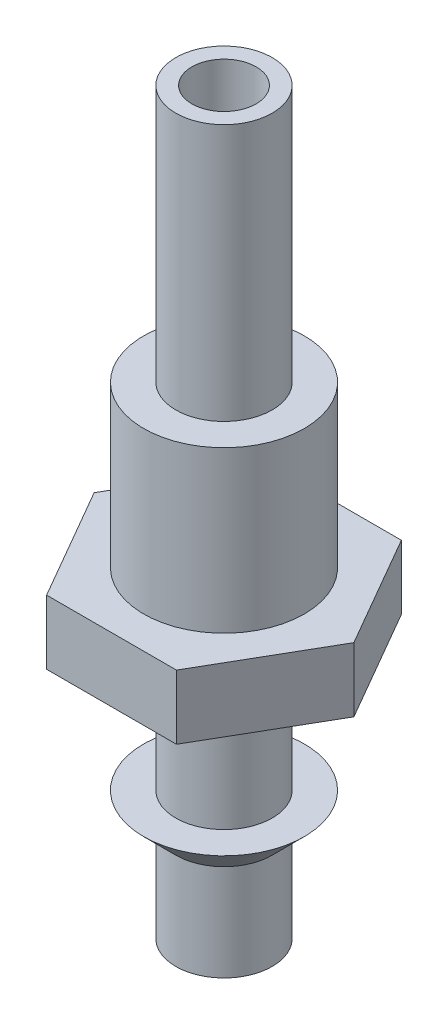
from build123d import *

# Parameters (mm, degrees)
HEX_7AF_DEPTH     = 2
BORE_PROFILE_2_R  = 1
FUEL_BORE_2_DEPTH = 24.613202522


with BuildPart() as part:
    # Lower Spigot Profile → Lower Spigot and Collar (revolve)
    with BuildSketch(Plane.XY, mode=Mode.PRIVATE) as lower_spigot_and_collar_sk:
        Polygon((0, 0), (0, -8), (1.5, -8), (1.5, -5), (2.5, -4), (1.5, -4), (1.5, 0), align=None)
    revolve(lower_spigot_and_collar_sk.sketch.rotate(Axis((0, 0, 0), (0, -1, 0)), 90), axis=Axis((0, 0, 0), (0, -1, 0)))

    # Hex Profile 7AF → Hex 7AF (add)
    with BuildSketch(Plane(origin=(0, 0, 0), x_dir=(1, 0, 0), z_dir=(0, 1, 0))):
        Polygon((4.041451884, 0), (2.020725942, 3.5), (-2.020725942, 3.5), (-4.041451884, 0), (-2.020725942, -3.5), (2.020725942, -3.5), align=None)
    extrude(amount=HEX_7AF_DEPTH)

    # Upper Pipe Profile → Upper Pipe (revolve)
    with BuildSketch(Plane.XY):
        Polygon((0, 2), (0, 15), (1.5, 15), (1.5, 7), (2.5, 7), (2.5, 2), align=None)
    revolve(axis=Axis((0, 2, 0), (0, 1, 0)))

    # Bore Profile Ø2 → Fuel Bore Ø2 (cut, through all)
    with BuildSketch(Plane(origin=(0, 15, 0), x_dir=(1, 0, 0), z_dir=(0, 1, 0))):
        with Locations(Location((0, 0, 0), (0, 0, 180))):
            Circle(BORE_PROFILE_2_R)
    extrude(amount=-FUEL_BORE_2_DEPTH, mode=Mode.SUBTRACT)


solid = part.part
